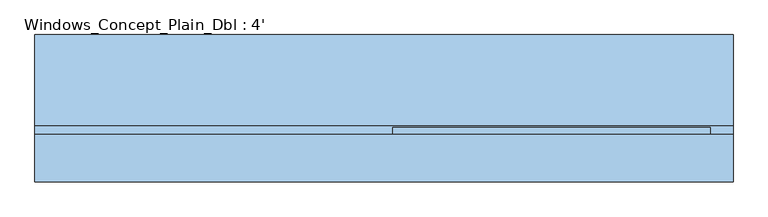
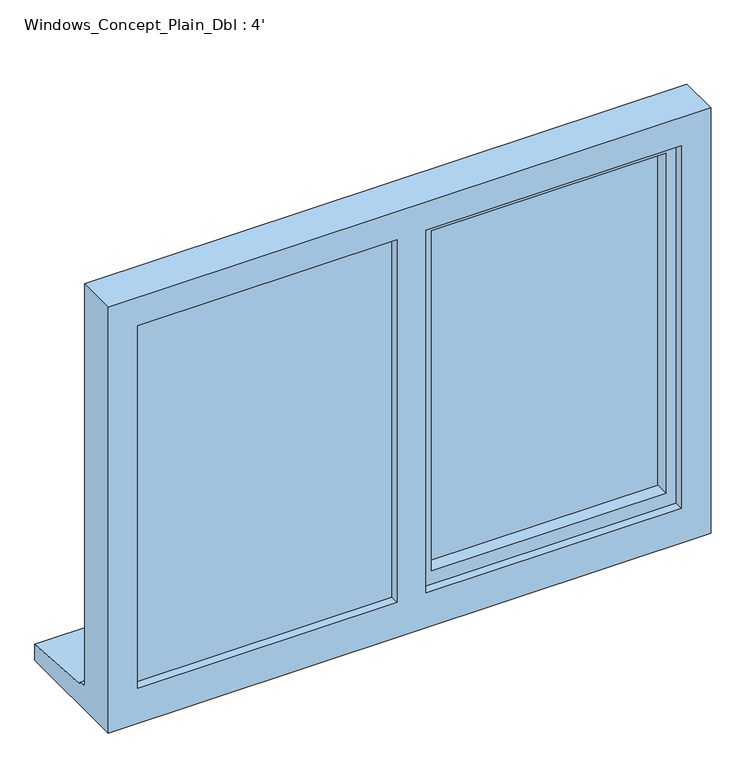
"""IFC4 building model written with IfcOpenShell, lengths in millimetres: window geometry, Windows_Concept_Plain_Dbl : 4'."""

from ifc_helpers import new_model, si_unit, frame, origin, place, context, project, spatial, polyline, outline, extrude, faceted_brep, source, transform, mapped, element, save


def windows_concept_plain_dbl_4_70a487c4(model_context):
    return source(origin(), model_context, "Body", "SolidModel", [
        faceted_brep([(-270.0, -42.9926322, 2070.0), (-270.0, 33.5543732, 2070.0), (-270.0, 33.5543732, 1263.0), (-270.0, -42.9926322, 1263.0), (-230.0, -13.9926322, 2030.0), (-230.0, -42.9926322, 2030.0), (-230.0, -42.9926322, 1303.0), (-230.0, -13.9926322, 1303.0), (-240.0, 10.0073678, 2040.0), (-240.0, -13.9926322, 2040.0), (-240.0, -13.9926322, 1293.0), (-240.0, 10.0073678, 1293.0), (-230.0, 33.5543732, 2030.0), (-230.0, 10.0073678, 2030.0), (-230.0, 10.0073678, 1303.0), (-230.0, 33.5543732, 1303.0), (284.6, 33.5543732, 1263.0), (284.6, -42.9926322, 1263.0), (244.6, -42.9926322, 1303.0), (244.6, -13.9926322, 1303.0), (254.6, -13.9926322, 1293.0), (254.6, 10.0073678, 1293.0), (244.6, 10.0073678, 1303.0), (244.6, 33.5543732, 1303.0), (284.6, 33.5543732, 2070.0), (284.6, -42.9926322, 2070.0), (244.6, -42.9926322, 2030.0), (244.6, -13.9926322, 2030.0), (254.6, -13.9926322, 2040.0), (254.6, 10.0073678, 2040.0), (244.6, 10.0073678, 2030.0), (244.6, 33.5543732, 2030.0)], [[[0, 1, 2, 3]], [[4, 5, 6, 7]], [[8, 9, 10, 11]], [[12, 13, 14, 15]], [[3, 2, 16, 17]], [[7, 6, 18, 19]], [[11, 10, 20, 21]], [[15, 14, 22, 23]], [[17, 16, 24, 25]], [[19, 18, 26, 27]], [[21, 20, 28, 29]], [[23, 22, 30, 31]], [[1, 24, 16, 2], [15, 23, 31, 12]], [[25, 24, 1, 0]], [[3, 17, 25, 0], [5, 26, 18, 6]], [[27, 26, 5, 4]], [[9, 28, 20, 10], [7, 19, 27, 4]], [[29, 28, 9, 8]], [[11, 21, 29, 8], [13, 30, 22, 14]], [[31, 30, 13, 12]]]),
        extrude(outline(polyline([(2050.0, -310.0), (2070.0, -310.0), (2070.0, -854.6), (1263.0, -854.6), (1263.0, -310.0), (1283.0, -310.0), (1283.0, -834.6), (2050.0, -834.6), (2050.0, -310.0)])), frame((0.0, -18.9926322, 0.0), z_axis=(0.0, 1.0, 0.0), x_axis=(0.0, 0.0, 1.0)), (0.0, 0.0, 1.0), 41.0),
        faceted_brep([(324.6, -60.9926322, 2110.0), (-894.6, -60.9926322, 2110.0), (-894.6, -60.9926322, 1200.0), (324.6, -60.9926322, 1200.0), (264.6, -60.9926322, 2050.0), (264.6, -60.9926322, 1275.0), (-252.0, -60.9926322, 1275.0), (-252.0, -60.9926322, 2050.0), (-310.0, -60.9926322, 2050.0), (-310.0, -60.9926322, 1275.0), (-834.6, -60.9926322, 1275.0), (-834.6, -60.9926322, 2050.0), (-894.6, 22.0073678, 2110.0), (-894.6, 22.0073678, 1251.0), (-894.6, 37.0073678, 1249.68767), (-894.6, 37.0073678, 1244.7449676), (-894.6, 195.9565678, 1233.8088847), (-894.6, 195.9565678, 1200.0), (324.6, 22.0073678, 2110.0), (324.6, 22.0073678, 1251.0), (-854.6, 22.0073678, 2070.0), (-854.6, 22.0073678, 1263.0), (-310.0, 22.0073678, 1263.0), (-310.0, 22.0073678, 2070.0), (-270.0, 22.0073678, 2070.0), (-270.0, 22.0073678, 1263.0), (284.6, 22.0073678, 1263.0), (284.6, 22.0073678, 2070.0), (-854.6, -42.9926322, 2070.0), (-854.6, -42.9926322, 1263.0), (-300.0, -42.9926322, 2070.0), (-300.0, -42.9926322, 1263.0), (-310.0, -42.9926322, 2050.0), (-834.6, -42.9926322, 2050.0), (-834.6, -42.9926322, 1275.0), (-310.0, -42.9926322, 1275.0), (-270.0, -42.9926322, 2070.0), (284.6, -42.9926322, 2070.0), (284.6, -42.9926322, 1263.0), (-270.0, -42.9926322, 1263.0), (264.6, -42.9926322, 2050.0), (-252.0, -42.9926322, 2050.0), (-252.0, -42.9926322, 1275.0), (264.6, -42.9926322, 1275.0), (-310.0, -18.9926322, 2070.0), (-300.0, -18.9926322, 2070.0), (324.6, 195.9565678, 1200.0), (324.6, 195.9565678, 1233.8088847), (324.6, 37.0073678, 1244.7449676), (324.6, 37.0073678, 1249.68767), (-300.0, -18.9926322, 1263.0), (-310.0, -18.9926322, 1263.0)], [[[0, 1, 2, 3], [4, 5, 6, 7], [8, 9, 10, 11]], [[2, 1, 12, 13, 14, 15, 16, 17]], [[13, 12, 18, 19], [20, 21, 22, 23], [24, 25, 26, 27]], [[21, 20, 28, 29]], [[28, 30, 31, 29], [32, 33, 34, 35]], [[36, 37, 38, 39], [40, 41, 42, 43]], [[33, 11, 10, 34]], [[1, 0, 18, 12]], [[28, 20, 23, 44, 45, 30]], [[27, 37, 36, 24]], [[11, 33, 32, 8]], [[40, 4, 7, 41]], [[19, 18, 0, 3, 46, 47, 48, 49]], [[27, 26, 38, 37]], [[4, 40, 43, 5]], [[45, 50, 31, 30]], [[50, 45, 44, 51]], [[51, 44, 23, 22]], [[25, 24, 36, 39]], [[41, 7, 6, 42]], [[8, 32, 35, 9]], [[46, 3, 2, 17]], [[47, 46, 17, 16]], [[48, 47, 16, 15]], [[49, 48, 15, 14]], [[19, 49, 14, 13]], [[22, 21, 29, 31, 50, 51]], [[26, 25, 39, 38]], [[6, 5, 43, 42]], [[35, 34, 10, 9]]]),
        extrude(outline(polyline([(-854.6, -18.9926322), (-300.0, -18.9926322), (-300.0, -42.9926322), (-854.6, -42.9926322), (-854.6, -18.9926322)])), frame((0.0, 0.0, 1263.0), z_axis=(0.0, 0.0, 1.0), x_axis=(1.0, 0.0, 0.0)), (0.0, 0.0, 1.0), 807.0),
        extrude(outline(polyline([(254.6, -13.9926322), (-240.0, -13.9926322), (-240.0, 10.0073678), (254.6, 10.0073678), (254.6, -13.9926322)])), frame((0.0, 0.0, 1293.0), z_axis=(0.0, 0.0, 1.0), x_axis=(1.0, 0.0, 0.0)), (0.0, 0.0, 1.0), 747.0),
    ])


if __name__ == "__main__":
    model = new_model("IFC4")
    model_context = context("Model", 3, world=origin())
    ifc_project = project(units=[si_unit("LENGTHUNIT", "METRE", prefix="MILLI")], contexts=[model_context])
    site = spatial("IfcSite", under=ifc_project)
    building = spatial("IfcBuilding", under=site)
    placement = place(None, origin())
    windows_concept_plain_dbl_4_shape = windows_concept_plain_dbl_4_70a487c4(model_context)
    element("IfcWindow", 1, ObjectType="Windows_Concept_Plain_Dbl : 4'", at=placement, inside=building, context=model_context, shape_type="MappedRepresentation", body=[
        mapped(windows_concept_plain_dbl_4_shape, transform((0.0, 0.0, 0.0), x_axis=(1.0, 0.0, 0.0), y_axis=(0.0, 1.0, 0.0), z_axis=(0.0, 0.0, 1.0))),
    ])
    save(model, "model.ifc")

# Revit data of these elements
# Type "Windows_Concept_Plain_Dbl : 4'"
#   Type Mark = "56"
#   Operation = "DoublePanelVertical"
#   Construction Type Id = "GSP4R"
#   Manufacturer = "Revit"
#   Keynote = "L10"
#   Analytic Construction = "1/8 in Pilkington single glazing"
#   Visual Light Transmittance = 0.9
#   Solar Heat Gain Coefficient = 0.78
#   Rough Width = 1219.2 mm
#   Rough Height = 910 mm
#   Height = 910 mm
#   Width = 1219.2 mm
#   Heat Transfer Coefficient (U) = 3.6886 W/(m²·K)
#   FrameOffset - External = 50 mm
#   Default Head Height = 2110 mm
#   Vis - Cavity Closers = yes
#   Define Thermal Properties by = 1
#   Material Trim = Window Frame
#   Material Glass = Glass
#   Material Frame = Window Frame
#   Wall Closure = (empty or 0)
# Element 1 (IfcWindow, "Windows_Concept_Plain_Dbl : 4'")
#   Materials on its faces: "Window Frame", "Glass"
# Materials
#   "Window Frame": colour RGB 249 249 249, transparency 0, Keynote = "L10", Cost = 0
#   "Glass": class "Glass", colour RGB 0 128 192, transparency 0.9, Description = "Soda Lime Glass", Cost = 0
